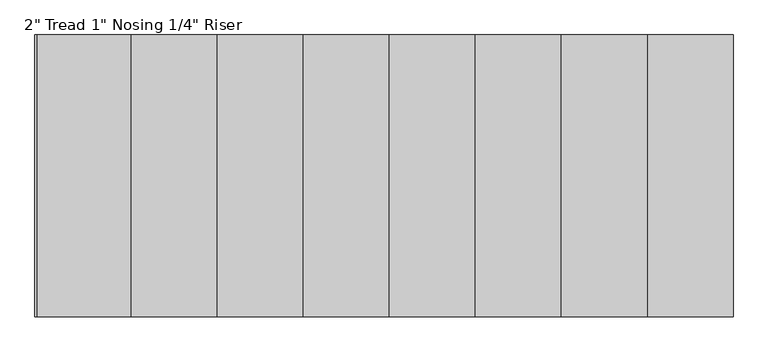
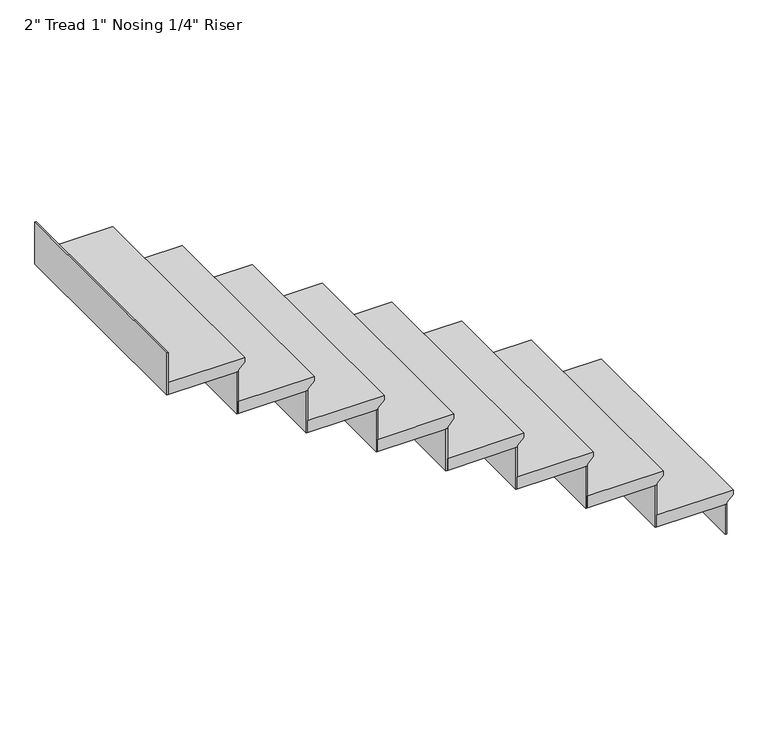
"""IFC4 building model written with IfcOpenShell, lengths in millimetres: stair flight geometry."""

from ifc_helpers import new_model, si_unit, origin, place, context, project, spatial, faceted_brep, source, transform, mapped, element, save


def stair_flight_934fe551(model_context):
    return source(origin(), model_context, "Body", "Brep", [
        faceted_brep([(-3247.3681702, -4870.057676, 158.75), (-3247.3681702, -4870.057676, 177.8), (-3247.3681702, -5784.457676, 177.8), (-3247.3681702, -5784.457676, 158.75), (-3272.7681702, -4870.057676, 133.35), (-3272.7681702, -5784.457676, 133.35), (-3552.1681702, -4870.057676, 177.8), (-3552.1681702, -5784.457676, 177.8), (-3272.7681702, -5784.457676, 127.0), (-3552.1681702, -5784.457676, 127.0), (-3552.1681702, -4870.057676, 127.0), (-3272.7681702, -4870.057676, 127.0)], [[[0, 1, 2, 3]], [[4, 0, 3, 5]], [[2, 1, 6, 7]], [[8, 9, 10, 11]], [[2, 7, 9, 8, 5, 3]], [[8, 11, 4, 5]], [[6, 1, 0, 4, 11, 10]], [[7, 6, 10, 9]]]),
        faceted_brep([(-3272.7681702, -4870.057676, 127.0), (-3272.7681702, -4870.057676, 0.0), (-3279.1181702, -4870.057676, 0.0), (-3279.1181702, -4870.057676, 127.0), (-3272.7681702, -5784.457676, 127.0), (-3279.1181702, -5784.457676, 127.0), (-3279.1181702, -5784.457676, 0.0), (-3272.7681702, -5784.457676, 0.0)], [[[0, 1, 2, 3]], [[4, 5, 6, 7]], [[1, 0, 4, 7]], [[2, 1, 7, 6]], [[3, 2, 6, 5]], [[0, 3, 5, 4]]]),
        faceted_brep([(-5507.9681702, -4870.057676, 1549.4), (-5507.9681702, -4870.057676, 1371.6), (-5514.3181702, -4870.057676, 1371.6), (-5514.3181702, -4870.057676, 1549.4), (-5507.9681702, -5784.457676, 1549.4), (-5514.3181702, -5784.457676, 1549.4), (-5514.3181702, -5784.457676, 1371.6), (-5507.9681702, -5784.457676, 1371.6)], [[[0, 1, 2, 3]], [[4, 5, 6, 7]], [[1, 0, 4, 7]], [[2, 1, 7, 6]], [[3, 2, 6, 5]], [[0, 3, 5, 4]]]),
        faceted_brep([(-3552.1681702, -4870.057676, 304.8), (-3552.1681702, -4870.057676, 127.0), (-3558.5181702, -4870.057676, 127.0), (-3558.5181702, -4870.057676, 304.8), (-3552.1681702, -5784.457676, 304.8), (-3558.5181702, -5784.457676, 304.8), (-3558.5181702, -5784.457676, 127.0), (-3552.1681702, -5784.457676, 127.0)], [[[0, 1, 2, 3]], [[4, 5, 6, 7]], [[1, 0, 4, 7]], [[2, 1, 7, 6]], [[3, 2, 6, 5]], [[0, 3, 5, 4]]]),
        faceted_brep([(-3526.7681702, -5784.457676, 355.6), (-3526.7681702, -4870.057676, 355.6), (-3831.5681702, -4870.057676, 355.6), (-3831.5681702, -5784.457676, 355.6), (-3552.1681702, -5784.457676, 304.8), (-3831.5681702, -5784.457676, 304.8), (-3831.5681702, -4870.057676, 304.8), (-3552.1681702, -4870.057676, 304.8), (-3552.1681702, -5784.457676, 311.15), (-3526.7681702, -5784.457676, 336.55), (-3552.1681702, -4870.057676, 311.15), (-3526.7681702, -4870.057676, 336.55)], [[[0, 1, 2, 3]], [[4, 5, 6, 7]], [[0, 3, 5, 4, 8, 9]], [[4, 7, 10, 8]], [[2, 1, 11, 10, 7, 6]], [[3, 2, 6, 5]], [[11, 1, 0, 9]], [[10, 11, 9, 8]]]),
        faceted_brep([(-3831.5681702, -4870.057676, 482.6), (-3831.5681702, -4870.057676, 304.8), (-3837.9181702, -4870.057676, 304.8), (-3837.9181702, -4870.057676, 482.6), (-3831.5681702, -5784.457676, 482.6), (-3837.9181702, -5784.457676, 482.6), (-3837.9181702, -5784.457676, 304.8), (-3831.5681702, -5784.457676, 304.8)], [[[0, 1, 2, 3]], [[4, 5, 6, 7]], [[1, 0, 4, 7]], [[2, 1, 7, 6]], [[3, 2, 6, 5]], [[0, 3, 5, 4]]]),
        faceted_brep([(-3806.1681702, -5784.457676, 533.4), (-3806.1681702, -4870.057676, 533.4), (-4110.9681702, -4870.057676, 533.4), (-4110.9681702, -5784.457676, 533.4), (-3831.5681702, -5784.457676, 482.6), (-4110.9681702, -5784.457676, 482.6), (-4110.9681702, -4870.057676, 482.6), (-3831.5681702, -4870.057676, 482.6), (-3831.5681702, -5784.457676, 488.95), (-3806.1681702, -5784.457676, 514.35), (-3831.5681702, -4870.057676, 488.95), (-3806.1681702, -4870.057676, 514.35)], [[[0, 1, 2, 3]], [[4, 5, 6, 7]], [[0, 3, 5, 4, 8, 9]], [[4, 7, 10, 8]], [[2, 1, 11, 10, 7, 6]], [[3, 2, 6, 5]], [[11, 1, 0, 9]], [[10, 11, 9, 8]]]),
        faceted_brep([(-4110.9681702, -4870.057676, 660.4), (-4110.9681702, -4870.057676, 482.6), (-4117.3181702, -4870.057676, 482.6), (-4117.3181702, -4870.057676, 660.4), (-4110.9681702, -5784.457676, 660.4), (-4117.3181702, -5784.457676, 660.4), (-4117.3181702, -5784.457676, 482.6), (-4110.9681702, -5784.457676, 482.6)], [[[0, 1, 2, 3]], [[4, 5, 6, 7]], [[1, 0, 4, 7]], [[2, 1, 7, 6]], [[3, 2, 6, 5]], [[0, 3, 5, 4]]]),
        faceted_brep([(-4085.5681702, -5784.457676, 711.2), (-4085.5681702, -4870.057676, 711.2), (-4390.3681702, -4870.057676, 711.2), (-4390.3681702, -5784.457676, 711.2), (-4110.9681702, -5784.457676, 660.4), (-4390.3681702, -5784.457676, 660.4), (-4390.3681702, -4870.057676, 660.4), (-4110.9681702, -4870.057676, 660.4), (-4110.9681702, -5784.457676, 666.75), (-4085.5681702, -5784.457676, 692.15), (-4110.9681702, -4870.057676, 666.75), (-4085.5681702, -4870.057676, 692.15)], [[[0, 1, 2, 3]], [[4, 5, 6, 7]], [[0, 3, 5, 4, 8, 9]], [[4, 7, 10, 8]], [[2, 1, 11, 10, 7, 6]], [[3, 2, 6, 5]], [[11, 1, 0, 9]], [[10, 11, 9, 8]]]),
        faceted_brep([(-4390.3681702, -4870.057676, 838.2), (-4390.3681702, -4870.057676, 660.4), (-4396.7181702, -4870.057676, 660.4), (-4396.7181702, -4870.057676, 838.2), (-4390.3681702, -5784.457676, 838.2), (-4396.7181702, -5784.457676, 838.2), (-4396.7181702, -5784.457676, 660.4), (-4390.3681702, -5784.457676, 660.4)], [[[0, 1, 2, 3]], [[4, 5, 6, 7]], [[1, 0, 4, 7]], [[2, 1, 7, 6]], [[3, 2, 6, 5]], [[0, 3, 5, 4]]]),
        faceted_brep([(-4364.9681702, -5784.457676, 889.0), (-4364.9681702, -4870.057676, 889.0), (-4669.7681702, -4870.057676, 889.0), (-4669.7681702, -5784.457676, 889.0), (-4390.3681702, -5784.457676, 838.2), (-4669.7681702, -5784.457676, 838.2), (-4669.7681702, -4870.057676, 838.2), (-4390.3681702, -4870.057676, 838.2), (-4390.3681702, -5784.457676, 844.55), (-4364.9681702, -5784.457676, 869.95), (-4390.3681702, -4870.057676, 844.55), (-4364.9681702, -4870.057676, 869.95)], [[[0, 1, 2, 3]], [[4, 5, 6, 7]], [[0, 3, 5, 4, 8, 9]], [[4, 7, 10, 8]], [[2, 1, 11, 10, 7, 6]], [[3, 2, 6, 5]], [[11, 1, 0, 9]], [[10, 11, 9, 8]]]),
        faceted_brep([(-4669.7681702, -4870.057676, 1016.0), (-4669.7681702, -4870.057676, 838.2), (-4676.1181702, -4870.057676, 838.2), (-4676.1181702, -4870.057676, 1016.0), (-4669.7681702, -5784.457676, 1016.0), (-4676.1181702, -5784.457676, 1016.0), (-4676.1181702, -5784.457676, 838.2), (-4669.7681702, -5784.457676, 838.2)], [[[0, 1, 2, 3]], [[4, 5, 6, 7]], [[1, 0, 4, 7]], [[2, 1, 7, 6]], [[3, 2, 6, 5]], [[0, 3, 5, 4]]]),
        faceted_brep([(-4644.3681702, -5784.457676, 1066.8), (-4644.3681702, -4870.057676, 1066.8), (-4949.1681702, -4870.057676, 1066.8), (-4949.1681702, -5784.457676, 1066.8), (-4669.7681702, -5784.457676, 1016.0), (-4949.1681702, -5784.457676, 1016.0), (-4949.1681702, -4870.057676, 1016.0), (-4669.7681702, -4870.057676, 1016.0), (-4669.7681702, -5784.457676, 1022.35), (-4644.3681702, -5784.457676, 1047.75), (-4669.7681702, -4870.057676, 1022.35), (-4644.3681702, -4870.057676, 1047.75)], [[[0, 1, 2, 3]], [[4, 5, 6, 7]], [[0, 3, 5, 4, 8, 9]], [[4, 7, 10, 8]], [[2, 1, 11, 10, 7, 6]], [[3, 2, 6, 5]], [[11, 1, 0, 9]], [[10, 11, 9, 8]]]),
        faceted_brep([(-4949.1681702, -4870.057676, 1193.8), (-4949.1681702, -4870.057676, 1016.0), (-4955.5181702, -4870.057676, 1016.0), (-4955.5181702, -4870.057676, 1193.8), (-4949.1681702, -5784.457676, 1193.8), (-4955.5181702, -5784.457676, 1193.8), (-4955.5181702, -5784.457676, 1016.0), (-4949.1681702, -5784.457676, 1016.0)], [[[0, 1, 2, 3]], [[4, 5, 6, 7]], [[1, 0, 4, 7]], [[2, 1, 7, 6]], [[3, 2, 6, 5]], [[0, 3, 5, 4]]]),
        faceted_brep([(-4923.7681702, -5784.457676, 1244.6), (-4923.7681702, -4870.057676, 1244.6), (-5228.5681702, -4870.057676, 1244.6), (-5228.5681702, -5784.457676, 1244.6), (-4949.1681702, -5784.457676, 1193.8), (-5228.5681702, -5784.457676, 1193.8), (-5228.5681702, -4870.057676, 1193.8), (-4949.1681702, -4870.057676, 1193.8), (-4949.1681702, -5784.457676, 1200.15), (-4923.7681702, -5784.457676, 1225.55), (-4949.1681702, -4870.057676, 1200.15), (-4923.7681702, -4870.057676, 1225.55)], [[[0, 1, 2, 3]], [[4, 5, 6, 7]], [[0, 3, 5, 4, 8, 9]], [[4, 7, 10, 8]], [[2, 1, 11, 10, 7, 6]], [[3, 2, 6, 5]], [[11, 1, 0, 9]], [[10, 11, 9, 8]]]),
        faceted_brep([(-5228.5681702, -4870.057676, 1371.6), (-5228.5681702, -4870.057676, 1193.8), (-5234.9181702, -4870.057676, 1193.8), (-5234.9181702, -4870.057676, 1371.6), (-5228.5681702, -5784.457676, 1371.6), (-5234.9181702, -5784.457676, 1371.6), (-5234.9181702, -5784.457676, 1193.8), (-5228.5681702, -5784.457676, 1193.8)], [[[0, 1, 2, 3]], [[4, 5, 6, 7]], [[1, 0, 4, 7]], [[2, 1, 7, 6]], [[3, 2, 6, 5]], [[0, 3, 5, 4]]]),
        faceted_brep([(-5203.1681702, -5784.457676, 1422.4), (-5203.1681702, -4870.057676, 1422.4), (-5482.5681702, -4870.057676, 1422.4), (-5507.9681702, -4870.057676, 1422.4), (-5507.9681702, -5784.457676, 1422.4), (-5228.5681702, -5784.457676, 1371.6), (-5507.9681702, -5784.457676, 1371.6), (-5507.9681702, -4870.057676, 1371.6), (-5482.5681702, -4870.057676, 1371.6), (-5228.5681702, -4870.057676, 1371.6), (-5228.5681702, -5784.457676, 1377.95), (-5203.1681702, -5784.457676, 1403.35), (-5228.5681702, -4870.057676, 1377.95), (-5203.1681702, -4870.057676, 1403.35)], [[[0, 1, 2, 3, 4]], [[5, 6, 7, 8, 9]], [[0, 4, 6, 5, 10, 11]], [[5, 9, 12, 10]], [[2, 1, 13, 12, 9, 8]], [[3, 2, 8, 7]], [[4, 3, 7, 6]], [[13, 1, 0, 11]], [[12, 13, 11, 10]]]),
    ])


if __name__ == "__main__":
    model = new_model("IFC4")
    model_context = context("Model", 3, world=origin())
    ifc_project = project(units=[si_unit("LENGTHUNIT", "METRE", prefix="MILLI")], contexts=[model_context])
    site = spatial("IfcSite", under=ifc_project)
    building = spatial("IfcBuilding", under=site)
    placement = place(None, origin())
    stair_flight_shape = stair_flight_934fe551(model_context)
    element("IfcStairFlight", 1, ObjectType="2\" Tread 1\" Nosing 1/4\" Riser", at=placement, inside=building, context=model_context, shape_type="MappedRepresentation", body=[
        mapped(stair_flight_shape, transform((0.0, 0.0, 0.0), x_axis=(1.0, 0.0, 0.0), y_axis=(0.0, 1.0, 0.0), z_axis=(0.0, 0.0, 1.0))),
    ])
    save(model, "model.ifc")
